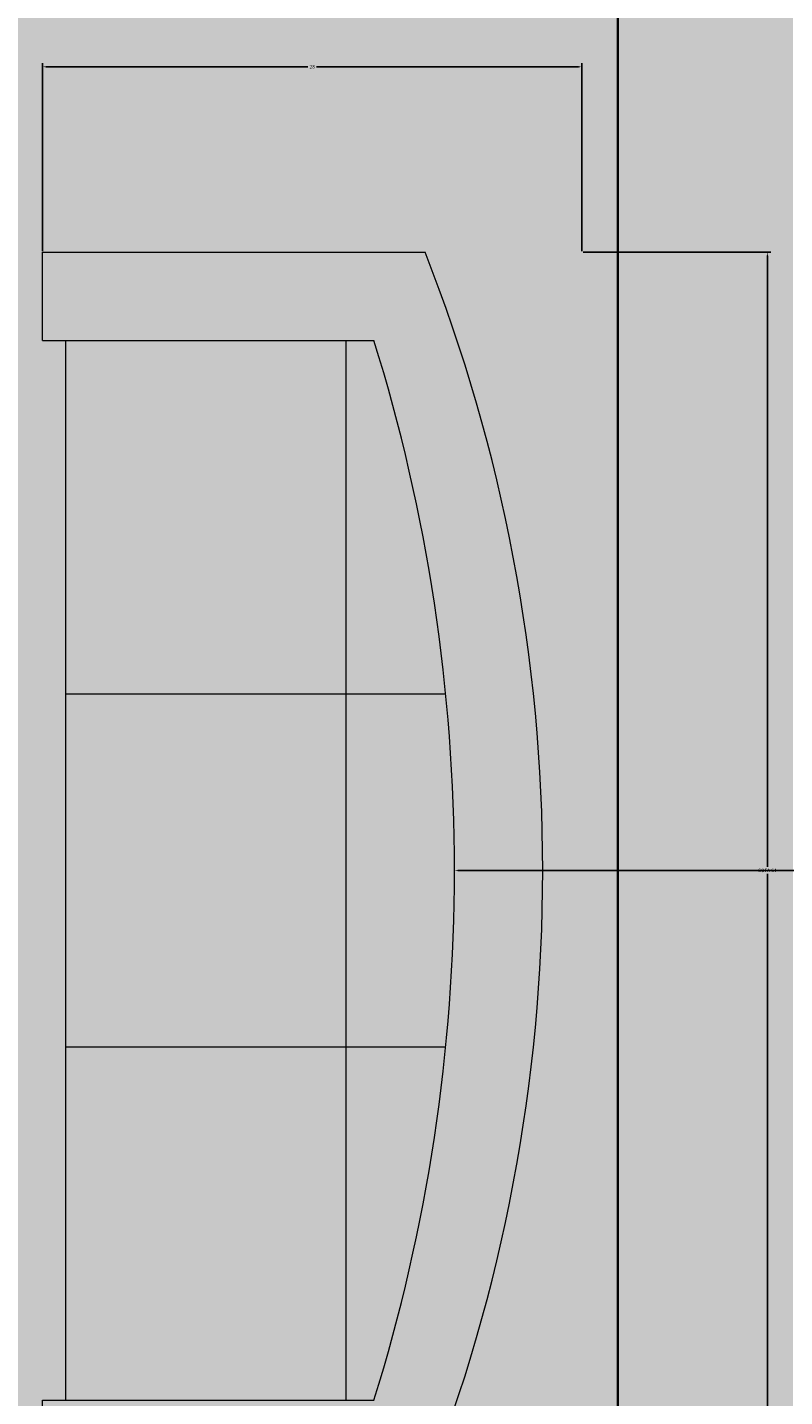
# Model space of a CAD drawing. Units: inches. Extents: x 3024 to 3952, y 1308 to 1863.
# Tile 19 of 29: x 3430 to 3469, y 1489 to 1559. Entities that reach past the tile are written whole.
import ezdxf

# ---------------------------------------------------------------- set-up
doc = ezdxf.new("R2010")
doc.units = ezdxf.units.IN
for name, color, linetype, lineweight in [('A-ANNO-DIMS', 2, 'Continuous', 18), ('A-FLOR-TILE-PATT', 7, 'Continuous', 13), ('A-FURN', 8, 'Continuous', 18), ('A-FURN-PATT', 9, 'Continuous', 13), ('A-WALL', 7, 'Continuous', 35)]:
    doc.layers.add(name, color=color, linetype=linetype, lineweight=lineweight)
doc.layers.add('A-FLOR-PATT', color=254, linetype='Continuous', lineweight=13, true_color=0xfeeab9)
doc.layers.add('A-WALL-PATT', color=254, linetype='Continuous', lineweight=13, true_color=0xcecce6)
doc.styles.get("Standard").update_dxf_attribs({"font": 'arial.ttf'})
doc.dimstyles.get("Standard").update_dxf_attribs({"dimtxt": 0.18, "dimasz": 0.18, "dimexe": 0.18, "dimexo": 0.0625, "dimgap": 0.09, "dimtad": 0, "dimtih": 1, "dimtoh": 1, "dimdec": 4, "dimzin": 0, "dimdsep": 46, "dimtxsty": 'Standard', "dimcen": 0.09, "dimadec": 0, "dimazin": 0, "dimtfac": 1, "dimtdec": 4, "dimtofl": 0, "dimtmove": 0, "dimatfit": 3, "dimfxl": 1, "dimtolj": 1, "dimtzin": 0, "dimarcsym": 0})

# ---------------------------------------------------------------- blocks, each defined once
blk = doc.blocks.new('Sofa - Roundback 7 ft.')
for p, q in [((-12.00002, -32.4421), (-12.00003, -6.5971)), ((11.99997, -32.4421), (11.99998, -6.5971)), ((-36.000027, -34), (-36.000027, -11.4696)), ((35.99998, -34), (35.99998, -11.4696)), ((-35.999844, -13.3819), (35.9998, -13.3819)), ((-36.000027, -32.4421), (35.99998, -32.4421))]:
    blk.add_line(p, q)
for points in [[(-36.000027, -34), (-42.000027, -34), (-42.000027, -8)], [(41.99998, -8), (41.99998, -34), (35.99998, -34)]]:
    blk.add_lwpolyline(points)
for centre, radius, start, end in [((0, -114.25), 114.25, 68.43141, 111.5686), ((-0.00001, -127.1968), 121.1968, 72.72033, 107.2797)]:
    blk.add_arc(centre, radius, start, end)
blk = doc.blocks.new('*D28')
at = {"layer": 'A-ANNO-DIMS', "color": 0, "lineweight": -2, "transparency": 16777216}
for p, q in [((3458.989, 1547.543), (3468.633, 1547.543)), ((3468.453, 1547.363), (3468.453, 1515.97)), ((3468.453, 1484.211), (3468.453, 1515.604)), ((3458.989, 1484.031), (3468.633, 1484.031))]:
    blk.add_line(p, q, dxfattribs=at)
at = {"layer": 'A-ANNO-DIMS', "color": 0, "transparency": 16777216}
for points in [[(3468.423, 1547.363), (3468.483, 1547.363), (3468.453, 1547.543)], [(3468.423, 1484.211), (3468.483, 1484.211), (3468.453, 1484.031)]]:
    blk.add_solid(points, dxfattribs=at)
at = {"layer": 'Defpoints', "color": 0, "transparency": 16777216}
for p in [(3458.926, 1547.543), (3458.926, 1484.031), (3468.453, 1484.031)]:
    blk.add_point(p, dxfattribs=at)
at = {"layer": 'A-ANNO-DIMS', "color": 0, "transparency": 16777216, "insert": (3468.453, 1515.787), "char_height": 0.18, "attachment_point": 5}
blk.add_mtext('\\A1;SOFA 64', dxfattribs=at)
blk = doc.blocks.new('*D29')
at = {"layer": 'A-ANNO-DIMS', "color": 0, "lineweight": -2, "transparency": 16777216}
for p, q in [((3431.203, 1547.605), (3431.203, 1557.25)), ((3431.383, 1557.07), (3444.844, 1557.07)), ((3458.746, 1557.07), (3445.285, 1557.07)), ((3458.926, 1547.605), (3458.926, 1557.25))]:
    blk.add_line(p, q, dxfattribs=at)
at = {"layer": 'A-ANNO-DIMS', "color": 0, "transparency": 16777216}
for points in [[(3431.383, 1557.1), (3431.383, 1557.04), (3431.203, 1557.07)], [(3458.746, 1557.1), (3458.746, 1557.04), (3458.926, 1557.07)]]:
    blk.add_solid(points, dxfattribs=at)
at = {"layer": 'Defpoints', "color": 0, "transparency": 16777216}
for p in [(3458.926, 1557.07), (3431.203, 1547.543), (3458.926, 1547.543)]:
    blk.add_point(p, dxfattribs=at)
at = {"layer": 'A-ANNO-DIMS', "color": 0, "transparency": 16777216, "insert": (3445.065, 1557.07), "char_height": 0.18, "attachment_point": 5}
blk.add_mtext('\\A1;28', dxfattribs=at)
blk = doc.blocks.new('*D104')
at = {"layer": 'A-ANNO-DIMS', "color": 0, "lineweight": -2, "transparency": 16777216}
for p, q in [((3360.648, 1515.787), (3360.828, 1515.787)), ((3360.738, 1515.697), (3360.738, 1515.877)), ((3507.355, 1515.787), (3452.554, 1515.787))]:
    blk.add_line(p, q, dxfattribs=at)
at = {"layer": 'A-ANNO-DIMS', "color": 0, "transparency": 16777216}
blk.add_solid([(3452.554, 1515.817), (3452.554, 1515.757), (3452.374, 1515.787)], dxfattribs=at)
at = {"layer": 'Defpoints', "color": 0, "transparency": 16777216}
for p in [(3360.738, 1515.787), (3452.374, 1515.787)]:
    blk.add_point(p, dxfattribs=at)
at = {"layer": 'A-ANNO-DIMS', "color": 0, "transparency": 16777216, "insert": (3507.835, 1515.787), "char_height": 0.18, "attachment_point": 5}
blk.add_mtext('\\A1;R91.64', dxfattribs=at)
blk = doc.blocks.new('*D105')
at = {"layer": 'A-ANNO-DIMS', "color": 0, "lineweight": -2, "transparency": 16777216}
for p, q in [((3370.437, 1515.787), (3370.617, 1515.787)), ((3370.527, 1515.697), (3370.527, 1515.877)), ((3508.74, 1515.787), (3457.09, 1515.787))]:
    blk.add_line(p, q, dxfattribs=at)
at = {"layer": 'A-ANNO-DIMS', "color": 0, "transparency": 16777216}
blk.add_solid([(3457.09, 1515.817), (3457.09, 1515.757), (3456.91, 1515.787)], dxfattribs=at)
at = {"layer": 'Defpoints', "color": 0, "transparency": 16777216}
for p in [(3370.527, 1515.787), (3456.91, 1515.787)]:
    blk.add_point(p, dxfattribs=at)
at = {"layer": 'A-ANNO-DIMS', "color": 0, "transparency": 16777216, "insert": (3509.22, 1515.787), "char_height": 0.18, "attachment_point": 5}
blk.add_mtext('\\A1;R86.38', dxfattribs=at)

msp = doc.modelspace()

# ---------------------------------------------------------------- hatches: boundary and pattern name
at = {"layer": 'A-FLOR-PATT', "transparency": 33554528}
h = msp.add_hatch(color=256, dxfattribs=at)
h.dxf.hatch_style = 1
h.paths.add_polyline_path([(3460.764, 1688.6064), (3412.764, 1688.6064), (3412.764, 1694.6064), (3460.764, 1694.6064), (3460.764, 1778.6064), (3406.764, 1778.6064), (3406.764, 1759.9514), (3318.2981, 1759.9514), (3318.2981, 1658.6064), (3322.5356, 1658.6064), (3322.5356, 1652.6064), (3292.764, 1652.6064), (3292.764, 1778.6064), (3106.764, 1778.6064), (3106.764, 1628.6064), (3172.764, 1628.6064), (3172.764, 1532.6064), (3166.764, 1532.6064), (3166.764, 1628.6064), (3106.764, 1628.6064), (3106.764, 1356.8452), (3202.812, 1356.8452), (3202.812, 1354.2534), (3202.812, 1353.8388), (3202.812, 1351.1212), (3202.812, 1347.8452), (3277.764, 1347.8452), (3277.764, 1353.8452), (3277.764, 1356.8452), (3277.764, 1442.6064), (3460.764, 1442.6064)])
h.paths.add_polyline_path([(3216.238, 1527.2064), (3216.238, 1491.2064), (3214.663, 1491.2064), (3214.663, 1491.2409, -0.3966224), (3180.243, 1526.6064), (3163.0285, 1526.6064), (3163.0285, 1531.1064), (3161.716, 1531.1064), (3161.716, 1561.1064), (3163.0285, 1561.1064), (3163.0285, 1531.1064), (3163.0285, 1526.6064), (3180.243, 1526.6064, 0.3966224), (3214.663, 1491.2409), (3214.663, 1527.2064)], flags=16)
h.paths.add_polyline_path([(3227.364, 1649.8972), (3191.364, 1649.8972), (3191.364, 1651.4722), (3227.364, 1651.4722)], flags=16)
h.paths.add_polyline_path([(3323.1172, 1606.7362), (3323.8545, 1606.8514), (3323.8545, 1594.8241), (3323.1172, 1594.9393)], flags=16)
h.paths.add_polyline_path([(3324.2232, 1606.909), (3330.1216, 1607.8307), (3330.1216, 1614.1093), (3339.3495, 1614.1093), (3340.2711, 1620.0078), (3352.4136, 1620.0078), (3353.3353, 1614.1093), (3359.9941, 1614.1093), (3360.9157, 1620.0078), (3373.0582, 1620.0078), (3373.9799, 1614.1093), (3383.2077, 1614.1093), (3383.2077, 1607.8307), (3389.1062, 1606.909), (3389.1062, 1594.7665), (3383.2077, 1593.8449), (3383.2077, 1587.5663), (3373.9799, 1587.5663), (3373.0583, 1581.6678), (3360.9157, 1581.6678), (3359.9941, 1587.5663), (3353.3353, 1587.5663), (3352.4136, 1581.6678), (3340.2711, 1581.6678), (3339.3495, 1587.5663), (3330.1216, 1587.5663), (3330.1216, 1593.8449), (3324.2232, 1594.7665)], flags=16)
h.paths.add_polyline_path([(3236.1584, 1693.1064), (3236.1584, 1723.1064), (3237.4709, 1723.1064), (3237.4709, 1693.1064)], flags=16)
h.paths.add_polyline_path([(3373.2158, 1600.6847), (3373.7965, 1600.7303), (3374.3268, 1600.7874), (3374.8132, 1600.8531), (3375.2621, 1600.9247), (3375.6801, 1600.9991), (3376.0736, 1601.0735), (3376.6855, 1601.19), (3377.366, 1601.3023), (3378.0667, 1601.3814), (3378.8026, 1601.4123), (3379.5865, 1601.3839), (3380.4537, 1601.2948), (3381.301, 1601.1717), (3382.0317, 1601.0433), (3382.4398, 1600.9607), (3382.6252, 1600.9201), (3382.919, 1600.8507), (3382.9044, 1600.8531), (3382.842, 1600.8678), (3382.7541, 1600.8896), (3382.6252, 1600.9201), (3382.4398, 1600.9607), (3382.1868, 1601.0119), (3381.8738, 1601.0711), (3381.5125, 1601.1346), (3381.1149, 1601.1988), (3380.6928, 1601.2601), (3380.2581, 1601.3149), (3379.8226, 1601.3597), (3379.3984, 1601.3908), (3378.9944, 1601.4054), (3378.6092, 1601.4042), (3378.2384, 1601.3886), (3377.8777, 1601.36), (3377.5227, 1601.32), (3377.1691, 1601.2698), (3376.8127, 1601.211), (3376.4491, 1601.145), (3376.0736, 1601.0735), (3375.4177, 1600.9494), (3374.5542, 1600.8119), (3373.5044, 1600.6988)], flags=0)
h.paths.add_polyline_path([(3380.0253, 1596.7351), (3380.499, 1596.6659), (3380.9706, 1596.6119), (3381.4375, 1596.5791), (3381.8971, 1596.5736), (3382.5886, 1596.6167), (3382.7848, 1596.6692), (3382.1465, 1596.5706), (3381.236, 1596.5815), (3380.3199, 1596.6865)], flags=0)
h.paths.add_polyline_path([(3369.6414, 1603.9617), (3370.1589, 1604.0021), (3370.6218, 1604.0539), (3371.0335, 1604.1173), (3371.3978, 1604.1921), (3371.7181, 1604.2785), (3371.9984, 1604.3761), (3372.2441, 1604.483), (3372.4611, 1604.5972), (3372.655, 1604.7163), (3372.8317, 1604.8384), (3372.9968, 1604.9611), (3373.3703, 1605.2455), (3373.8426, 1605.5328), (3374.4624, 1605.7539), (3375.1058, 1605.8302), (3375.7221, 1605.8261), (3376.4109, 1605.76), (3377.1534, 1605.6376), (3377.8945, 1605.473), (3378.1382, 1605.409), (3377.7394, 1605.5074), (3377.3509, 1605.5937), (3376.9704, 1605.6677), (3376.5999, 1605.7288), (3376.2417, 1605.7762), (3375.8979, 1605.8092), (3375.5707, 1605.8271), (3375.2621, 1605.8291), (3374.9745, 1605.8146), (3374.7092, 1605.7832), (3374.4647, 1605.7359), (3374.239, 1605.6742), (3374.0298, 1605.5996), (3373.835, 1605.5134), (3373.6525, 1605.4171), (3373.4801, 1605.3123), (3373.3156, 1605.2002), (3373.1562, 1605.0825), (3372.7603, 1604.781), (3372.236, 1604.4588), (3371.5738, 1604.2283), (3370.8493, 1604.0794), (3369.9262, 1603.976)], flags=0)
h.paths.add_polyline_path([(3366.7533, 1606.5832), (3367.1713, 1606.5519), (3367.5378, 1606.5374), (3367.8568, 1606.5394), (3368.1325, 1606.5573), (3368.3694, 1606.5903), (3368.5717, 1606.6377), (3368.7438, 1606.6988), (3368.89, 1606.7728), (3369.0146, 1606.8591), (3369.121, 1606.9568), (3369.2094, 1607.0646), (3369.2792, 1607.181), (3369.3295, 1607.3046), (3369.3596, 1607.4339), (3369.3688, 1607.5676), (3369.3565, 1607.7042), (3369.3218, 1607.8422), (3369.2649, 1607.9804), (3369.1893, 1608.1187), (3369.0993, 1608.2569), (3368.9992, 1608.3952), (3368.8934, 1608.5334), (3368.7861, 1608.6717), (3368.6817, 1608.8099), (3368.4212, 1609.1804), (3368.2685, 1609.7106), (3368.4883, 1610.1814), (3369.0537, 1610.4604), (3369.6717, 1610.5097), (3370.2812, 1610.3612), (3370.4805, 1610.2968), (3370.1882, 1610.3839), (3369.9284, 1610.4472), (3369.6905, 1610.4842), (3369.4662, 1610.4933), (3369.2555, 1610.4765), (3369.0608, 1610.4367), (3368.884, 1610.3767), (3368.7274, 1610.2994), (3368.5931, 1610.2077), (3368.4833, 1610.1045), (3368.4002, 1609.9927), (3368.3451, 1609.8747), (3368.3166, 1609.7517), (3368.3127, 1609.6244), (3368.331, 1609.4935), (3368.3696, 1609.3597), (3368.4261, 1609.2237), (3368.4985, 1609.0863), (3368.5845, 1608.9482), (3368.6817, 1608.8099), (3368.7861, 1608.6717), (3368.8934, 1608.5334), (3368.9992, 1608.3952), (3369.0993, 1608.2569), (3369.3398, 1607.8876), (3369.3941, 1607.2896), (3368.9774, 1606.7817), (3368.3928, 1606.5742), (3367.7162, 1606.5303), (3367.0044, 1606.5585)], flags=0)
h.paths.add_polyline_path([(3362.1859, 1610.2589), (3362.5478, 1610.2845), (3362.8348, 1610.3275), (3363.0585, 1610.3863), (3363.2303, 1610.4595), (3363.3619, 1610.5457), (3363.463, 1610.6432), (3363.5376, 1610.7502), (3363.5876, 1610.8643), (3363.6153, 1610.9834), (3363.6229, 1611.1055), (3363.6125, 1611.2283), (3363.5861, 1611.3496), (3363.5462, 1611.4673), (3363.4949, 1611.5797), (3363.4358, 1611.6871), (3363.3723, 1611.7902), (3363.3081, 1611.8897), (3363.2468, 1611.9863), (3363.192, 1612.0808), (3363.0258, 1612.4261), (3363.3371, 1612.8672), (3363.9008, 1612.9782), (3364.4822, 1612.9641), (3365.1098, 1612.9074), (3365.328, 1612.8805), (3364.9615, 1612.9208), (3364.6426, 1612.9496), (3364.3668, 1612.9669), (3364.1299, 1612.9726), (3363.9276, 1612.9669), (3363.7555, 1612.9496), (3363.6093, 1612.9208), (3363.4848, 1612.8805), (3363.3782, 1612.8289), (3363.2889, 1612.7672), (3363.2169, 1612.6969), (3363.1622, 1612.6193), (3363.1247, 1612.5361), (3363.1046, 1612.4484), (3363.1017, 1612.358), (3363.1161, 1612.266), (3363.1472, 1612.1738), (3363.192, 1612.0808), (3363.2468, 1611.9863), (3363.3081, 1611.8897), (3363.3723, 1611.7902), (3363.4358, 1611.6871), (3363.6363, 1611.323), (3363.5979, 1610.7003), (3363.0863, 1610.3651), (3362.3983, 1610.2622)], flags=0)
h.paths.add_polyline_path([(3352.356, 1581.2991), (3352.2408, 1580.5618), (3340.4439, 1580.5618), (3340.3287, 1581.2991)], flags=16)
h.paths.add_polyline_path([(3340.4439, 1621.1137), (3352.2408, 1621.1137), (3352.356, 1620.3764), (3340.3287, 1620.3764)], flags=16)
h.paths.add_polyline_path([(3278.4282, 1504.7424), (3290.3831, 1504.7424), (3290.3831, 1502.7499), (3291.0473, 1502.7499), (3291.0473, 1494.7799), (3290.3831, 1494.7799), (3290.3831, 1494.1158), (3291.0473, 1494.1158), (3291.0473, 1486.1458), (3290.3831, 1486.1458), (3290.3831, 1484.1533), (3291.0473, 1484.1533), (3291.0473, 1483.4892, -0.0909091), (3291.0473, 1468.8776), (3291.0473, 1468.2135), (3290.3831, 1468.2135), (3290.3831, 1464.8926), (3278.4282, 1464.8926), (3278.4282, 1472.8626), (3277.764, 1473.5268), (3277.764, 1478.84), (3278.4282, 1479.5042)], flags=16)
h.paths.add_polyline_path([(3278.7603, 1504.4103), (3290.051, 1504.4103), (3290.051, 1465.2247), (3278.7603, 1465.2247)], flags=0)
h.paths.add_polyline_path([(3123.904, 1600.7821), (3117.9039, 1602.7821), (3117.9039, 1599.7821), (3119.4039, 1599.7821), (3119.4039, 1596.7821), (3118.4039, 1596.7821), (3118.4039, 1598.7821), (3117.9039, 1598.7821), (3117.9039, 1596.2821), (3109.9039, 1596.2821), (3109.9039, 1617.2821), (3117.9039, 1617.2821), (3117.9039, 1610.7821), (3123.9038, 1612.7821, -0.7025712), (3137.9039, 1606.7822, -0.7025621)], flags=16)
h.paths.add_polyline_path([(3123.9039, 1602.7822), (3123.9039, 1610.7822, -0.7345333), (3136.9039, 1606.7822, -0.7345297)], flags=0)
h.paths.add_polyline_path([(3177.972, 1689.6473), (3109.2405, 1689.6473), (3109.2405, 1741.1959), (3177.972, 1741.1959)], flags=16)
h.paths.add_polyline_path([(3373.0006, 1581.2991), (3372.8854, 1580.5618), (3361.0885, 1580.5618), (3360.9733, 1581.2991)], flags=16)
h.paths.add_polyline_path([(3361.0885, 1621.1137), (3372.8854, 1621.1137), (3373.0006, 1620.3764), (3360.9733, 1620.3764)], flags=16)
h.paths.add_polyline_path([(3116.9039, 1598.2821, -0.4142136), (3116.1539, 1597.2821), (3111.9039, 1597.2821, -0.4142136), (3110.9039, 1598.0321), (3110.9039, 1615.2821, -0.4142136), (3111.6539, 1616.2821), (3115.9039, 1616.2821, -0.4142136), (3116.9039, 1615.5321)], flags=0)
h.paths.add_polyline_path([(3121.6122, 1728.1369), (3121.6122, 1696.5205), (3110.2715, 1696.5205), (3110.2715, 1714.3906), (3121.6122, 1714.3906), (3121.6122, 1716.4526), (3110.2715, 1716.4526), (3110.2715, 1734.3228), (3123.3304, 1734.3228), (3123.3304, 1729.8552), (3134.6711, 1741.1959), (3134.6711, 1728.1369)], flags=0)
h.paths.add_polyline_path([(3389.4748, 1606.8514), (3390.2122, 1606.7362), (3390.2122, 1594.9393), (3389.4748, 1594.8241)], flags=16)
h.paths.add_polyline_path([(3257.6842, 1762.8281), (3259.6842, 1768.8281), (3256.6842, 1768.8281), (3256.6842, 1767.3281), (3253.6842, 1767.3281), (3253.6842, 1768.3281), (3255.6842, 1768.3281), (3255.6842, 1768.8281), (3253.1842, 1768.8281), (3253.1842, 1776.8281), (3274.1842, 1776.8281), (3274.1842, 1768.8281), (3267.6842, 1768.8281), (3269.6842, 1762.8282, -0.7025712), (3263.6843, 1748.8282, -0.7025621)], flags=16)
h.paths.add_polyline_path([(3259.6842, 1762.8281), (3267.6843, 1762.8281, -0.7345333), (3263.6842, 1749.8282, -0.7345297)], flags=0)
h.paths.add_polyline_path([(3411.264, 1715.6064), (3411.264, 1716.9189), (3441.264, 1716.9189), (3441.264, 1715.6064)], flags=16)
h.paths.add_polyline_path([(3178.3806, 1449.1876), (3178.3806, 1397.639), (3109.6491, 1397.639), (3109.6491, 1449.1876)], flags=16)
h.paths.add_polyline_path([(3397.1501, 1541.7146), (3419.6183, 1541.7146), (3419.6183, 1496.7783), (3397.1501, 1496.7783)], flags=16)
h.paths.add_polyline_path([(3254.1842, 1770.5781), (3254.1842, 1774.8281, -0.4142136), (3254.9342, 1775.8281), (3272.1842, 1775.8281, -0.4142136), (3273.1842, 1775.0781), (3273.1842, 1770.8281, -0.4142136), (3272.4342, 1769.8281), (3255.1842, 1769.8281, -0.4142136)], flags=0)
h.paths.add_polyline_path([(3403.672, 1500.7601), (3403.6016, 1500.3997), (3403.5328, 1500.0441), (3403.4662, 1499.6867), (3403.4027, 1499.3226), (3403.3464, 1498.9532), (3403.3025, 1498.5811), (3403.2759, 1498.2091), (3403.2714, 1497.8401), (3403.3064, 1497.2813), (3403.3491, 1497.1219), (3403.2689, 1497.6395), (3403.2778, 1498.3719), (3403.3635, 1499.0984), (3403.4889, 1499.8168), (3403.6016, 1500.3997), (3403.672, 1500.7601), (3403.744, 1501.1315), (3403.817, 1501.5205), (3403.891, 1501.9336), (3403.9656, 1502.3769), (3404.0404, 1502.8572), (3404.115, 1503.3786), (3404.2264, 1504.2311), (3404.2571, 1504.5223), (3404.1552, 1503.6598), (3404.0063, 1502.6193), (3403.8604, 1501.7518), (3403.744, 1501.1315)], flags=0)
h.paths.add_polyline_path([(3406.5868, 1505.0416), (3406.6121, 1504.5236), (3406.6492, 1504.0526), (3406.6956, 1503.624), (3406.7491, 1503.2333), (3406.8072, 1502.8759), (3406.8676, 1502.5473), (3406.9281, 1502.243), (3407.0268, 1501.7597), (3407.1416, 1501.1368), (3407.2087, 1500.3904), (3407.1804, 1499.6703), (3407.1078, 1498.9956), (3407.0074, 1498.3199), (3406.8809, 1497.6059), (3406.7403, 1496.9627), (3406.7418, 1496.9824), (3406.7491, 1497.0249), (3406.8229, 1497.3409), (3406.8364, 1497.4025), (3406.878, 1497.6078), (3406.9261, 1497.8614), (3406.9777, 1498.1526), (3407.0298, 1498.4712), (3407.0797, 1498.8068), (3407.1243, 1499.149), (3407.1607, 1499.4874), (3407.1859, 1499.8115), (3407.1978, 1500.1137), (3407.1969, 1500.3962), (3407.1841, 1500.6642), (3407.1609, 1500.9225), (3407.1284, 1501.1761), (3407.0876, 1501.43), (3407.0398, 1501.6891), (3406.9862, 1501.9585), (3406.8832, 1502.4628), (3406.7712, 1503.0713), (3406.6657, 1503.8424), (3406.5924, 1504.7735)], flags=0)
h.paths.add_polyline_path([(3409.2517, 1507.8962), (3409.2752, 1507.4282), (3409.3079, 1507.0076), (3409.3501, 1506.6314), (3409.4015, 1506.2969), (3409.4624, 1506.0009), (3409.5326, 1505.7406), (3409.6119, 1505.5128), (3409.6988, 1505.3131), (3409.7915, 1505.1368), (3409.8883, 1504.9792), (3409.9875, 1504.8356), (3410.0872, 1504.7015), (3410.1859, 1504.572), (3410.4508, 1504.2132), (3410.7205, 1503.6035), (3410.8059, 1502.8824), (3410.7619, 1502.0875), (3410.6122, 1501.2299), (3410.4402, 1500.6169), (3410.2538, 1500.0031), (3410.0536, 1499.3219), (3409.9909, 1499.0812), (3410.1761, 1499.7472), (3410.3596, 1500.3513), (3410.4512, 1500.6561), (3410.5312, 1500.9412), (3410.6013, 1501.226), (3410.6614, 1501.512), (3410.7111, 1501.7964), (3410.7496, 1502.0763), (3410.7764, 1502.3489), (3410.7909, 1502.6114), (3410.7926, 1502.8608), (3410.7808, 1503.0944), (3410.7553, 1503.31), (3410.7169, 1503.5087), (3410.6667, 1503.6921), (3410.6061, 1503.8621), (3410.5361, 1504.0203), (3410.4578, 1504.1686), (3410.3726, 1504.3088), (3410.2815, 1504.4424), (3410.1859, 1504.572), (3410.0872, 1504.7015), (3409.859, 1505.0083), (3409.5943, 1505.5117), (3409.4266, 1506.1336), (3409.324, 1506.8011), (3409.2586, 1507.6407)], flags=0)
h.paths.add_polyline_path([(3411.4914, 1510.5878), (3411.4432, 1510.1586), (3411.4054, 1509.775), (3411.38, 1509.4354), (3411.3681, 1509.1376), (3411.3698, 1508.8784), (3411.3843, 1508.6542), (3411.4112, 1508.4618), (3411.4497, 1508.2974), (3411.4994, 1508.1575), (3411.5595, 1508.0388), (3411.6296, 1507.9375), (3411.7097, 1507.851), (3411.802, 1507.7792), (3411.9096, 1507.7225), (3412.0353, 1507.6817), (3412.1821, 1507.6572), (3412.3528, 1507.6496), (3412.5505, 1507.6597), (3412.778, 1507.6879), (3413.0364, 1507.7341), (3413.3194, 1507.7955), (3413.6188, 1507.8687), (3413.9264, 1507.95), (3414.234, 1508.036), (3414.5333, 1508.1232), (3414.8163, 1508.208), (3415.0747, 1508.287), (3415.3023, 1508.3569), (3415.5007, 1508.4158), (3415.6733, 1508.4617), (3416.1158, 1508.5538), (3416.512, 1508.2591), (3416.716, 1507.6581), (3416.61, 1507.0003), (3416.3052, 1506.3411), (3415.8928, 1505.618), (3415.7339, 1505.3633), (3415.9914, 1505.791), (3416.201, 1506.1583), (3416.3666, 1506.4739), (3416.4925, 1506.7462), (3416.5828, 1506.9838), (3416.6413, 1507.1949), (3416.6725, 1507.3883), (3416.6799, 1507.5705), (3416.6662, 1507.7417), (3416.6339, 1507.9), (3416.5851, 1508.0436), (3416.5223, 1508.1709), (3416.4478, 1508.28), (3416.3639, 1508.3692), (3416.273, 1508.4368), (3416.1765, 1508.4815), (3416.0718, 1508.5047), (3415.9553, 1508.5079), (3415.8237, 1508.493), (3415.6733, 1508.4617), (3415.5007, 1508.4158), (3415.3327, 1508.3659), (3414.6495, 1508.157), (3414.0606, 1507.9855), (3413.4456, 1507.8229), (3412.8838, 1507.701), (3412.5505, 1507.6597), (3412.0748, 1507.6354), (3411.595, 1507.8883), (3411.398, 1508.4429), (3411.3624, 1508.9927), (3411.3854, 1509.5711), (3411.4578, 1510.3071)], flags=0)
h.paths.add_polyline_path([(3135.0797, 1449.1876), (3135.0797, 1436.1286), (3122.0208, 1436.1286), (3122.0208, 1404.5122), (3110.6801, 1404.5122), (3110.6801, 1422.3823), (3122.0208, 1422.3823), (3122.0208, 1424.4443), (3110.6801, 1424.4443), (3110.6801, 1442.3145), (3123.739, 1442.3145), (3123.739, 1437.8469)], flags=0)
h.paths.add_polyline_path([(3416.4944, 1514.2949), (3416.4837, 1513.8511), (3416.4893, 1513.4867), (3416.5102, 1513.1926), (3416.5451, 1512.9593), (3416.5929, 1512.7775), (3416.6524, 1512.6379), (3416.7224, 1512.531), (3416.8017, 1512.4488), (3416.8886, 1512.3882), (3416.9813, 1512.3476), (3417.0781, 1512.3251), (3417.1773, 1512.3189), (3417.277, 1512.3274), (3417.3757, 1512.3488), (3417.4713, 1512.3813), (3417.5627, 1512.4229), (3417.65, 1512.471), (3417.7338, 1512.5225), (3417.8146, 1512.5747), (3417.8931, 1512.6245), (3417.9699, 1512.6691), (3418.2968, 1512.8265), (3418.6505, 1512.4645), (3418.7037, 1511.9342), (3418.6693, 1511.3839), (3418.6076, 1510.8228), (3418.5777, 1510.5927), (3418.6197, 1510.9333), (3418.6525, 1511.2311), (3418.6759, 1511.4903), (3418.6899, 1511.7144), (3418.6946, 1511.9069), (3418.6899, 1512.0713), (3418.6759, 1512.2112), (3418.6525, 1512.33), (3418.6197, 1512.4311), (3418.5778, 1512.5177), (3418.5276, 1512.5903), (3418.4705, 1512.6488), (3418.4075, 1512.6933), (3418.3399, 1512.7237), (3418.2686, 1512.7401), (3418.1951, 1512.7424), (3418.1204, 1512.7307), (3418.0455, 1512.7055), (3417.9792, 1512.6736), (3417.65, 1512.471), (3417.5627, 1512.4229), (3417.4713, 1512.3813), (3417.3757, 1512.3488), (3417.277, 1512.3274), (3416.878, 1512.2936), (3416.5757, 1512.7549), (3416.492, 1513.3145), (3416.4808, 1514.0384)], flags=0)
h.paths.add_polyline_path([(3392.8223, 1481.9454), (3396.7707, 1481.9454), (3396.7707, 1480.9201), (3428.3585, 1480.9201), (3428.3585, 1481.9454), (3432.3069, 1481.9454), (3432.3069, 1464.8354, -0.266667), (3392.8223, 1464.8354)], flags=16)
h.paths.add_polyline_path([(3431.203, 1547.5428), (3450.8613, 1547.5428, -0.1904762), (3450.8614, 1484.031), (3431.203, 1484.031), (3431.203, 1488.5675), (3432.3809, 1488.5675), (3432.3809, 1543.0062), (3431.203, 1543.0062)], flags=16)
h.paths.add_polyline_path([(3451.9233, 1524.86, -0.0496282), (3451.9233, 1506.7138), (3446.7921, 1506.7138), (3446.7921, 1524.86)], flags=0)
h.paths.add_polyline_path([(3460.764, 1436.6064), (3277.764, 1436.6064), (3277.764, 1356.8452), (3277.764, 1353.8452), (3460.764, 1353.8452)], flags=17)
h.paths.add_polyline_path([(3121.3033, 1577.378), (3153.693, 1577.378), (3153.693, 1586.6752), (3121.3033, 1586.6752)], flags=24)
h.paths.add_polyline_path([(3164.1457, 1464.1276), (3210.4801, 1464.1276), (3210.4801, 1473.4247), (3164.1457, 1473.4247)], flags=24)
h.paths.add_polyline_path([(3343.1909, 1505.8863), (3373.7236, 1505.8863), (3373.7236, 1515.1773), (3343.1909, 1515.1773)], flags=24)
h.paths.add_polyline_path([(3337.6353, 1564.2926), (3370.0189, 1564.2926), (3370.0189, 1573.5836), (3337.6353, 1573.5836)], flags=24)
h.paths.add_polyline_path([(3419.204, 1753.8578), (3453.3997, 1753.8578), (3453.3997, 1762.9956), (3419.204, 1762.9956)], flags=24)
h.paths.add_polyline_path([(3341.2523, 1701.0246), (3381.0761, 1701.0246), (3381.0761, 1710.3156), (3341.2523, 1710.3156)], flags=24)
h.paths.add_polyline_path([(3245.8895, 1726.2997), (3278.2793, 1726.2997), (3278.2793, 1735.5968), (3245.8895, 1735.5968)], flags=24)
h.paths.add_polyline_path([(3128.8045, 1668.6736), (3175.1389, 1668.6736), (3175.1389, 1677.9707), (3128.8045, 1677.9707)], flags=24)
h.paths.add_polyline_path([(3345.9997, 1396.0062), (3389.09, 1396.0062), (3389.09, 1405.3033), (3345.9997, 1405.3033)], flags=24)
at = {"layer": 'A-FLOR-TILE-PATT', "transparency": 33554569}
h = msp.add_hatch(dxfattribs=at)
h.set_pattern_fill('ANGLE', color=256, scale=2)
h.set_pattern_definition([(0, (0, 0), (0, 13.97), [10.16, -3.81]), (90, (0, 0), (-13.97, 9e-16), [10.16, -3.81])])
h.paths.add_polyline_path([(3292.764, 1778.6064), (3232.764, 1778.6064), (3232.764, 1694.6064), (3236.1584, 1694.6064), (3236.1584, 1723.1064), (3237.4709, 1723.1064), (3237.4709, 1723.0777, -0.3870039), (3266.1209, 1694.6064), (3292.764, 1694.6064)])
h.paths.add_polyline_path([(3263.6843, 1748.8282, -0.7025621), (3257.6842, 1762.8281), (3259.6842, 1768.8281), (3256.6842, 1768.8281), (3256.6842, 1767.3281), (3253.6842, 1767.3281), (3253.6842, 1768.3281), (3255.6842, 1768.3281), (3255.6842, 1768.8281), (3253.1842, 1768.8281), (3253.1842, 1776.8281), (3274.1842, 1776.8281), (3274.1842, 1768.8281), (3267.6842, 1768.8281), (3269.6842, 1762.8282, -0.7025712)], flags=16)
h.paths.add_polyline_path([(3263.6842, 1749.8282, -0.7345297), (3259.6842, 1762.8281), (3267.6843, 1762.8281, -0.7345333)], flags=0)
h.paths.add_polyline_path([(3255.1842, 1769.8281, -0.4142136), (3254.1842, 1770.5781), (3254.1842, 1774.8281, -0.4142136), (3254.9342, 1775.8281), (3272.1842, 1775.8281, -0.4142136), (3273.1842, 1775.0781), (3273.1842, 1770.8281, -0.4142136), (3272.4342, 1769.8281)], flags=0)
h.paths.add_polyline_path([(3460.764, 1436.6064), (3277.764, 1436.6064), (3277.764, 1356.8452), (3277.764, 1353.8452), (3460.764, 1353.8452)])
h.paths.add_polyline_path([(3166.764, 1628.6064), (3106.764, 1628.6064), (3106.764, 1532.6064), (3133.066, 1532.6064, -0.3870039), (3161.716, 1561.0777), (3161.716, 1561.1064), (3163.0285, 1561.1064), (3163.0285, 1532.6064), (3166.764, 1532.6064)])
h.paths.add_polyline_path([(3123.904, 1600.7821), (3117.9039, 1602.7821), (3117.9039, 1599.7821), (3119.4039, 1599.7821), (3119.4039, 1596.7821), (3118.4039, 1596.7821), (3118.4039, 1598.7821), (3117.9039, 1598.7821), (3117.9039, 1596.2821), (3109.9039, 1596.2821), (3109.9039, 1617.2821), (3117.9039, 1617.2821), (3117.9039, 1610.7821), (3123.9038, 1612.7821, -0.7025712), (3137.9039, 1606.7822, -0.7025621)], flags=16)
h.paths.add_polyline_path([(3123.9039, 1602.7822), (3123.9039, 1610.7822, -0.7345333), (3136.9039, 1606.7822, -0.7345297)], flags=0)
h.paths.add_polyline_path([(3116.1539, 1597.2821), (3111.9039, 1597.2821, -0.4142136), (3110.9039, 1598.0321), (3110.9039, 1615.2821, -0.4142136), (3111.6539, 1616.2821), (3115.9039, 1616.2821, -0.4142136), (3116.9039, 1615.5321), (3116.9039, 1598.2821, -0.4142136)], flags=0)
h.paths.add_polyline_path([(3245.8895, 1726.2997), (3278.2793, 1726.2997), (3278.2793, 1735.5968), (3245.8895, 1735.5968)], flags=24)
h.paths.add_polyline_path([(3345.9997, 1396.0062), (3389.09, 1396.0062), (3389.09, 1405.3033), (3345.9997, 1405.3033)], flags=24)
h.paths.add_polyline_path([(3121.3033, 1577.378), (3153.693, 1577.378), (3153.693, 1586.6752), (3121.3033, 1586.6752)], flags=24)
at = {"layer": 'A-FURN-PATT', "transparency": 33554600}
h = msp.add_hatch(color=256, dxfattribs=at)
h.dxf.hatch_style = 1
h.paths.add_polyline_path([(3450.8613, 1547.5428), (3431.203, 1547.5428), (3431.203, 1543.0062), (3448.2376, 1543.0062, -0.1519478), (3448.2376, 1488.5675), (3431.203, 1488.5675), (3431.203, 1484.031), (3450.8614, 1484.031, 0.1904762)])
h.paths.add_polyline_path([(3446.7921, 1543.0062), (3432.3809, 1543.0062), (3432.3809, 1524.86), (3446.7921, 1524.86)], flags=17)
h.paths.add_polyline_path([(3448.2376, 1543.0062), (3446.7921, 1543.0062), (3446.7921, 1524.86), (3451.9233, 1524.86, 0.0506466)], flags=17)
h.paths.add_polyline_path([(3446.7921, 1524.86), (3432.3809, 1524.86), (3432.3809, 1506.7138), (3446.7921, 1506.7138)], flags=17)
h.paths.add_polyline_path([(3451.9233, 1524.86), (3446.7921, 1524.86), (3446.7921, 1506.7138), (3451.9233, 1506.7138, 0.0496282)], flags=17)
h.paths.add_polyline_path([(3446.7921, 1506.7138), (3432.3809, 1506.7138), (3432.3809, 1488.5675), (3446.7921, 1488.5675)], flags=17)
h.paths.add_polyline_path([(3451.9233, 1506.7138), (3446.7921, 1506.7138), (3446.7921, 1488.5675), (3448.2376, 1488.5675, 0.0506467)], flags=17)
h.paths.add_polyline_path([(3428.3585, 1480.9201), (3412.5646, 1480.9201), (3412.5646, 1468.377), (3428.3585, 1468.377)], flags=17)
h.paths.add_polyline_path([(3412.5646, 1480.9201), (3396.7707, 1480.9201), (3396.7707, 1468.377), (3412.5646, 1468.377)], flags=17)
h.paths.add_polyline_path([(3396.7707, 1481.9454), (3392.8223, 1481.9454), (3392.8223, 1464.8354, 0.266667), (3432.3069, 1464.8354), (3432.3069, 1481.9454), (3428.3585, 1481.9454), (3428.3585, 1467.119, -0.2279232), (3396.7707, 1467.119)])
h.paths.add_polyline_path([(3428.3585, 1467.119), (3428.3585, 1468.377), (3412.5646, 1468.377), (3412.5646, 1463.5192, 0.1125187)], flags=17)
h.paths.add_polyline_path([(3412.5646, 1468.377), (3396.7707, 1468.377), (3396.7707, 1467.119, 0.1125189), (3412.5646, 1463.5192)], flags=17)
at = {"layer": 'A-WALL-PATT'}
h = msp.add_hatch(color=256, dxfattribs=at)
h.dxf.hatch_style = 1
h.paths.add_polyline_path([(3106.764, 1778.6064), (3140.5977, 1778.6064), (3140.5977, 1781.8824), (3140.5977, 1784.6), (3140.5977, 1787.6064), (3097.764, 1787.6064), (3097.764, 1590.213), (3101.04, 1590.213), (3103.7576, 1590.213), (3106.764, 1590.213)])
h.paths.add_polyline_path([(3253.5314, 1781.8824), (3253.5314, 1784.6), (3253.5314, 1787.6064), (3194.6826, 1787.6064), (3194.6826, 1785.0146), (3194.6826, 1784.6), (3194.6826, 1781.8824), (3194.6826, 1778.6064), (3253.5314, 1778.6064)])
h.paths.add_polyline_path([(3333.856, 1782.2838), (3333.856, 1784.7474), (3333.856, 1787.6064), (3272.0523, 1787.6064), (3272.0523, 1785.0146), (3272.0523, 1784.6), (3272.0523, 1781.8824), (3272.0523, 1778.6064), (3333.856, 1778.6064)])
h.paths.add_polyline_path([(3428.8344, 1784.6), (3428.8344, 1787.6064), (3378.3947, 1787.6064), (3378.3947, 1784.7474), (3378.3947, 1782.2838), (3378.3947, 1778.6064), (3428.8344, 1778.6064), (3428.8344, 1781.8824)], flags=17)
h.paths.add_polyline_path([(3469.764, 1787.6064), (3451.9386, 1787.6064), (3451.9386, 1785.0146), (3451.9386, 1784.6), (3451.9386, 1781.8824), (3451.9386, 1778.6064), (3460.764, 1778.6064), (3460.764, 1353.8452), (3277.764, 1353.8452), (3277.764, 1347.8452), (3469.764, 1347.8452), (3469.764, 1353.8452)])
h.paths.add_polyline_path([(3106.764, 1571.6922), (3104.1722, 1571.6922), (3103.7576, 1571.6922), (3101.04, 1571.6922), (3097.764, 1571.6922), (3097.764, 1347.8452), (3148.7271, 1347.8452), (3148.7271, 1351.1212), (3148.7271, 1353.8388), (3148.7271, 1356.8452), (3106.764, 1356.8452)])
h.paths.add_polyline_path([(3277.764, 1532.6064), (3262.7605, 1532.6064), (3262.7605, 1582.9359), (3256.7605, 1582.9359), (3256.7605, 1532.6064), (3244.2116, 1532.6064), (3216.238, 1532.6064), (3216.238, 1527.2064), (3216.238, 1526.6064), (3271.764, 1526.6064), (3271.764, 1356.8452), (3202.812, 1356.8452), (3202.812, 1354.2534), (3202.812, 1353.8388), (3202.812, 1351.1212), (3202.812, 1347.8452), (3277.764, 1347.8452), (3277.764, 1353.8452), (3277.764, 1356.8452)])
h.paths.add_polyline_path([(3180.238, 1532.6064), (3163.0285, 1532.6064), (3163.0285, 1531.1064), (3163.0285, 1526.6064), (3180.243, 1526.6064, -0.0041669), (3180.238, 1527.2064)])
h.paths.add_polyline_path([(3133.0285, 1531.1064, -0.0125059), (3133.066, 1532.6064), (3106.764, 1532.6064), (3106.764, 1526.6064), (3133.0285, 1526.6064)], flags=17)
h.paths.add_polyline_path([(3172.764, 1628.6064), (3166.764, 1628.6064), (3166.764, 1532.6064), (3172.764, 1532.6064)])
h.paths.add_polyline_path([(3232.764, 1649.8972), (3227.364, 1649.8972), (3226.764, 1649.8972), (3226.764, 1634.6064), (3106.764, 1634.6064), (3106.764, 1628.6064), (3232.764, 1628.6064)])

# ---------------------------------------------------------------- linework, layer by layer
at = {"layer": 'A-WALL'}
msp.add_line((3460.764, 1353.8452), (3460.764, 1778.6064), dxfattribs=at)

# ---------------------------------------------------------------- block references
at = {"layer": 'A-FURN', "xscale": 0.75609235024942, "yscale": 0.75609235024942, "zscale": 0.75609235024942, "rotation": 270}
msp.add_blockref('Sofa - Roundback 7 ft.', (3456.9101, 1515.7869), dxfattribs=at)

# ---------------------------------------------------------------- dimensions: what is measured, and where the dimension line sits
at = {"layer": 'A-ANNO-DIMS'}
dim = msp.add_linear_dim(base=(3458.9263, 1557.0695), p1=(3431.203, 1547.5428), p2=(3458.9263, 1547.5428), dimstyle='Standard', override={"dimdec": 0, "dimlfac": 1, "dimrnd": 0, "dimzin": 0, "dimdsep": 46, "dimlunit": 2}, dxfattribs=at)
dim.commit()
dim.dimension.update_dxf_attribs({"geometry": '*D29', "text_midpoint": (3445.0647, 1557.0695)})
dim = msp.add_linear_dim(base=(3468.4531, 1484.031), p1=(3458.9263, 1547.5428), p2=(3458.9263, 1484.031), angle=270, text='SOFA <>', dimstyle='Standard', override={"dimdec": 0, "dimlfac": 1, "dimrnd": 0, "dimzin": 0, "dimdsep": 46, "dimlunit": 2}, dxfattribs=at)
dim.commit()
dim.dimension.update_dxf_attribs({"geometry": '*D28', "text_midpoint": (3468.4531, 1515.7869)})
for center, mpoint, picture, middle in [((3360.7376, 1515.7869), (3452.3735, 1515.787), '*D104', (3507.3551, 1515.7871)), ((3370.5265, 1515.7869), (3456.9101, 1515.787), '*D105', (3508.7402, 1515.7871))]:
    dim = msp.add_radius_dim(center=center, mpoint=mpoint, dimstyle='Standard', override={"dimdec": 2, "dimlfac": 1, "dimrnd": 0, "dimzin": 0, "dimdsep": 46, "dimlunit": 2}, dxfattribs=at)
    dim.commit()
    dim.dimension.update_dxf_attribs({"geometry": picture, "text_midpoint": middle, "dimtype": 164})

doc.saveas('drawing.dxf')
